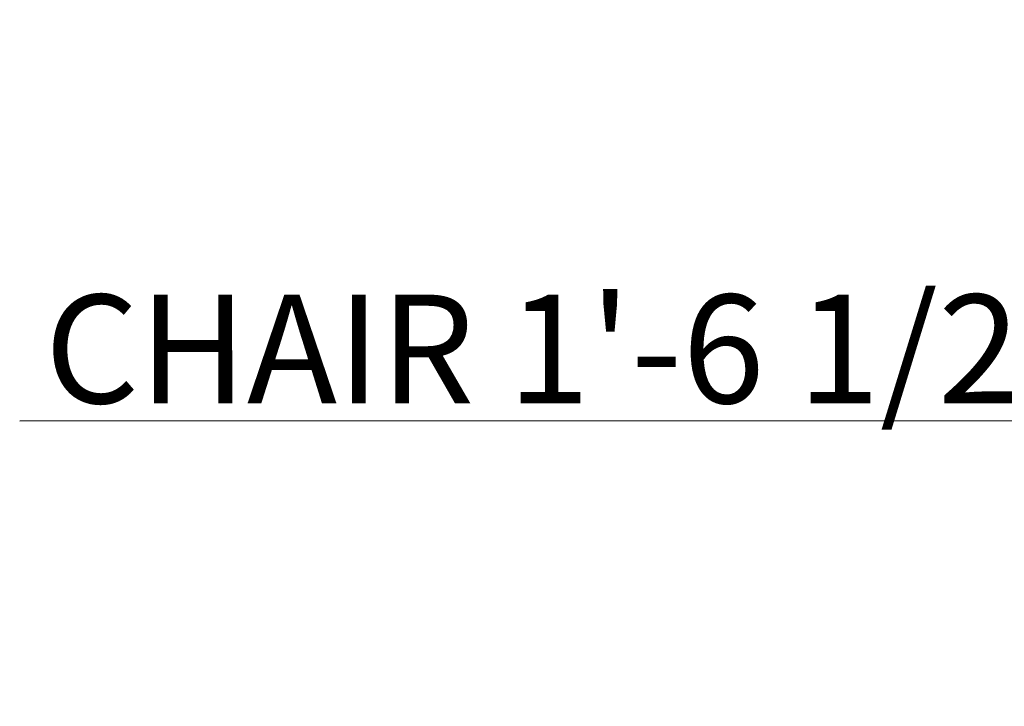
# Model space of a CAD drawing. Units: inches. Extents: x 1102 to 2414, y 295 to 1561.
# Tile 1 of 11: x 1102 to 1429, y 797 to 1025. Entities that reach past the tile are written whole.
import ezdxf

# ---------------------------------------------------------------- set-up
doc = ezdxf.new("R2010")
doc.units = ezdxf.units.IN
doc.layers.add('A-ANNO-DIMS', color=2, linetype='Continuous', lineweight=18)
doc.styles.get("Standard").update_dxf_attribs({"font": 'arial.ttf'})
doc.dimstyles.new('ISO-25', dxfattribs={"dimtxt": 36, "dimasz": 24, "dimexe": 1.25, "dimexo": 0.625, "dimtad": 1, "dimlunit": 4, "dimtxsty": 'Standard', "dimcen": 2.5, "dimadec": 0, "dimazin": 0, "dimtfac": 1, "dimtmove": 0, "dimatfit": 3, "dimfxl": 1, "dimarcsym": 0})

# ---------------------------------------------------------------- blocks, each defined once
blk = doc.blocks.new('*D17')
at = {"layer": 'A-ANNO-DIMS', "color": 0, "lineweight": -2, "transparency": 16777216}
for p, q in [((1600.9, 891.85), (1102.3, 891.8)), ((1624.9, 893.98), (1624.9, 890.6)), ((1643.27, 891.85), (1624.9, 891.85)), ((1643.27, 893.98), (1643.27, 890.6)), ((1667.27, 891.85), (1691.27, 891.85))]:
    blk.add_line(p, q, dxfattribs=at)
at = {"layer": 'A-ANNO-DIMS', "color": 0, "transparency": 16777216}
for points in [[(1600.9, 895.85), (1600.9, 887.85), (1624.9, 891.85)], [(1667.27, 895.85), (1667.27, 887.85), (1643.27, 891.85)]]:
    blk.add_solid(points, dxfattribs=at)
at = {"layer": 'Defpoints', "color": 0, "transparency": 16777216}
for p in [(1624.9, 894.6), (1624.9, 891.85), (1643.27, 894.6)]:
    blk.add_point(p, dxfattribs=at)
at = {"layer": 'A-ANNO-DIMS', "color": 0, "transparency": 16777216, "insert": (1339.6, 911.06), "char_height": 36, "attachment_point": 5, "rotation": 0.0057}
blk.add_mtext('CHAIR 1\'-6 1/2" TYP.', dxfattribs=at)

msp = doc.modelspace()

# ---------------------------------------------------------------- dimensions: what is measured, and where the dimension line sits
at = {"layer": 'A-ANNO-DIMS'}
dim = msp.add_linear_dim(base=(1624.9, 891.848), p1=(1643.269, 894.605), p2=(1624.9, 894.603), angle=180.00567, text='CHAIR <> TYP.', dimstyle='ISO-25', override={"dimdec": 1, "dimlfac": 1, "dimrnd": 0, "dimzin": 1, "dimdsep": 46, "dimlunit": 4, "dimfrac": 2}, dxfattribs=at)
dim.commit()
dim.dimension.update_dxf_attribs({"geometry": '*D17', "text_midpoint": (1339.596, 911.058)})

doc.saveas('drawing.dxf')
